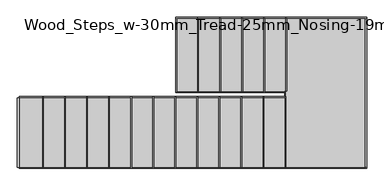
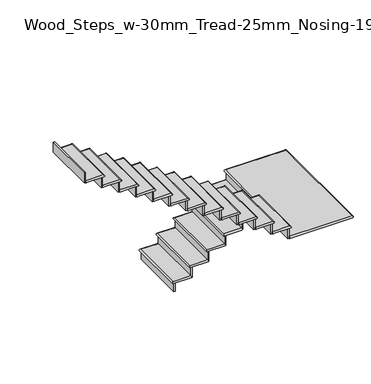
"""IFC4 building model written with IfcOpenShell, lengths in millimetres: stair flight geometry, Wood_Steps_w-30mm_Tread-25mm_Nosing-19mm_Riser."""

from ifc_helpers import new_model, si_unit, frame, origin, place, context, project, spatial, circle_curve, ellipse_curve, faceted_brep, source, transform, mapped, element, save
from ifc_brep_helpers import plane_surface, cylinder_surface, advanced_brep


def wood_steps_w_30mm_tread_25mm_nosing_19mm_riser_1d491615(model_context):
    return source(origin(), model_context, "Body", "SolidModel", [
        advanced_brep(
        [(-8665.149573, -11058.3255223, 3708.88), (-8665.149573, -11058.3255223, 3738.88), (-8665.149573, -10219.6521308, 3738.88), (-8665.149573, -10219.6521308, 3708.88), (-8400.9545789, -11058.3255223, 3738.88), (-8400.9545789, -10219.6521308, 3738.88), (-8400.9545789, -10219.6521308, 3708.88), (-8400.9545789, -11058.3255223, 3708.88)],
        [
            (0, 1, ellipse_curve(frame((-8665.149573, -11058.3255223, 3723.88), z_axis=(-0.7071067811865475, 0.7071067811865475, 0.0), x_axis=(-0.7071067811865474, -0.7071067811865476, 0.0)), 21.2132034, 15.0)),
            (1, 2),
            (2, 3, ellipse_curve(frame((-8665.149573, -10219.6521308, 3723.88), z_axis=(-0.7071067811865475, -0.7071067811865475, 0.0), x_axis=(0.7071067811865474, -0.7071067811865476, 0.0)), 21.2132034, 15.0)),
            (3, 0),
            (4, 5),
            (5, 2),
            (1, 4),
            (6, 7),
            (7, 0),
            (3, 6),
            (4, 7, circle_curve(frame((-8400.9545789, -11058.3255223, 3723.88), z_axis=(1.0, 0.0, 0.0), x_axis=(0.0, 1.0, 0.0)), 15.0)),
            (6, 5, circle_curve(frame((-8400.9545789, -10219.6521308, 3723.88), z_axis=(1.0, 0.0, 0.0), x_axis=(0.0, -1.0, 0.0)), 15.0)),
        ],
        [
            cylinder_surface(frame((-8665.149573, -11058.3255223, 3723.88), z_axis=(0.0, -1.0, 0.0), x_axis=(1.0, 0.0, 0.0)), 15.0),
            plane_surface(frame((-6495.4132565, -10219.6521308, 3738.88), z_axis=(0.0, 0.0, 1.0), x_axis=(-1.0, 0.0, 0.0))),
            plane_surface(frame((-6495.4132565, -10219.6521308, 3708.88), z_axis=(0.0, 0.0, -1.0), x_axis=(1.0, 0.0, 0.0))),
            plane_surface(frame((-8400.9545789, -11058.3255223, 3738.88), z_axis=(1.0, 0.0, 0.0), x_axis=(0.0, 0.0, -1.0))),
            cylinder_surface(frame((-8400.9545789, -11058.3255223, 3723.88), z_axis=(1.0, 0.0, 0.0), x_axis=(0.0, 1.0, 0.0)), 15.0),
            cylinder_surface(frame((-8665.149573, -10219.6521308, 3723.88), z_axis=(-1.0, 0.0, 0.0), x_axis=(0.0, -1.0, 0.0)), 15.0),
        ],
        [
            (0, [[1, 2, 3, 4]]),
            (1, [[5, 6, -2, 7]]),
            (2, [[8, 9, -4, 10]]),
            (3, [[-5, 11, -8, 12]]),
            (4, [[-11, -7, -1, -9]]),
            (5, [[-3, -6, -12, -10]]),
        ],
    ),
        faceted_brep([(-8655.149573, -11058.3255223, 3708.88), (-8655.149573, -11058.3255223, 3576.32), (-8636.149573, -11058.3255223, 3576.32), (-8636.149573, -11058.3255223, 3708.88), (-8655.149573, -10219.6521308, 3708.88), (-8636.149573, -10219.6521308, 3708.88), (-8636.149573, -10219.6521308, 3576.32), (-8655.149573, -10219.6521308, 3576.32)], [[[0, 1, 2, 3]], [[4, 5, 6, 7]], [[1, 0, 4, 7]], [[2, 1, 7, 6]], [[3, 2, 6, 5]], [[0, 3, 5, 4]]]),
        faceted_brep([(-8400.9545789, -11058.3255223, 3871.44), (-8400.9545789, -11058.3255223, 3708.88), (-8381.9545789, -11058.3255223, 3708.88), (-8381.9545789, -11058.3255223, 3871.44), (-8400.9545789, -10219.6521308, 3871.44), (-8381.9545789, -10219.6521308, 3871.44), (-8381.9545789, -10219.6521308, 3708.88), (-8400.9545789, -10219.6521308, 3708.88)], [[[0, 1, 2, 3]], [[4, 5, 6, 7]], [[1, 0, 4, 7]], [[2, 1, 7, 6]], [[3, 2, 6, 5]], [[0, 3, 5, 4]]]),
        advanced_brep(
        [(-8146.7595849, -11058.3255223, 3901.44), (-8146.7595849, -10219.6521308, 3901.44), (-8410.9545789, -10219.6521308, 3901.44), (-8410.9545789, -11058.3255223, 3901.44), (-8146.7595849, -10219.6521308, 3871.44), (-8146.7595849, -11058.3255223, 3871.44), (-8410.9545789, -11058.3255223, 3871.44), (-8410.9545789, -10219.6521308, 3871.44)],
        [
            (0, 1),
            (1, 2),
            (2, 3),
            (3, 0),
            (4, 5),
            (5, 6),
            (6, 7),
            (7, 4),
            (0, 5, circle_curve(frame((-8146.7595849, -11058.3255223, 3886.44), z_axis=(1.0, 0.0, 0.0), x_axis=(0.0, 1.0, 0.0)), 15.0)),
            (4, 1, circle_curve(frame((-8146.7595849, -10219.6521308, 3886.44), z_axis=(1.0, 0.0, 0.0), x_axis=(0.0, -1.0, 0.0)), 15.0)),
            (6, 3, ellipse_curve(frame((-8410.9545789, -11058.3255223, 3886.44), z_axis=(-0.7071067811865475, 0.7071067811865475, 0.0), x_axis=(-0.7071067811865474, -0.7071067811865476, 0.0)), 21.2132034, 15.0)),
            (2, 7, ellipse_curve(frame((-8410.9545789, -10219.6521308, 3886.44), z_axis=(-0.7071067811865475, -0.7071067811865475, 0.0), x_axis=(0.7071067811865474, -0.7071067811865476, 0.0)), 21.2132034, 15.0)),
        ],
        [
            plane_surface(frame((-6495.4132565, -10219.6521308, 3901.44), z_axis=(0.0, 0.0, 1.0), x_axis=(-1.0, 0.0, 0.0))),
            plane_surface(frame((-6495.4132565, -10219.6521308, 3871.44), z_axis=(0.0, 0.0, -1.0), x_axis=(1.0, 0.0, 0.0))),
            plane_surface(frame((-8146.7595849, -11058.3255223, 3901.44), z_axis=(1.0, 0.0, 0.0), x_axis=(0.0, 0.0, -1.0))),
            cylinder_surface(frame((-8410.9545789, -11058.3255223, 3886.44), z_axis=(0.0, -1.0, 0.0), x_axis=(1.0, 0.0, 0.0)), 15.0),
            cylinder_surface(frame((-8146.7595849, -11058.3255223, 3886.44), z_axis=(1.0, 0.0, 0.0), x_axis=(0.0, 1.0, 0.0)), 15.0),
            cylinder_surface(frame((-8410.9545789, -10219.6521308, 3886.44), z_axis=(-1.0, 0.0, 0.0), x_axis=(0.0, -1.0, 0.0)), 15.0),
        ],
        [
            (0, [[1, 2, 3, 4]]),
            (1, [[5, 6, 7, 8]]),
            (2, [[-1, 9, -5, 10]]),
            (3, [[11, -3, 12, -7]]),
            (4, [[-9, -4, -11, -6]]),
            (5, [[-12, -2, -10, -8]]),
        ],
    ),
        faceted_brep([(-8146.7595849, -11058.3255223, 4034.0), (-8146.7595849, -11058.3255223, 3871.44), (-8127.7595849, -11058.3255223, 3871.44), (-8127.7595849, -11058.3255223, 4034.0), (-8146.7595849, -10219.6521308, 4034.0), (-8127.7595849, -10219.6521308, 4034.0), (-8127.7595849, -10219.6521308, 3871.44), (-8146.7595849, -10219.6521308, 3871.44)], [[[0, 1, 2, 3]], [[4, 5, 6, 7]], [[1, 0, 4, 7]], [[2, 1, 7, 6]], [[3, 2, 6, 5]], [[0, 3, 5, 4]]]),
        advanced_brep(
        [(-7893.1206135, -11058.3255223, 4064.0), (-7893.1206135, -10219.6521308, 4064.0), (-8156.7595849, -10219.6521308, 4064.0), (-8156.7595849, -11058.3255223, 4064.0), (-7893.1206135, -10219.6521308, 4034.0), (-7893.1206135, -11058.3255223, 4034.0), (-8156.7595849, -11058.3255223, 4034.0), (-8156.7595849, -10219.6521308, 4034.0)],
        [
            (0, 1),
            (1, 2),
            (2, 3),
            (3, 0),
            (4, 5),
            (5, 6),
            (6, 7),
            (7, 4),
            (0, 5, circle_curve(frame((-7893.1206135, -11058.3255223, 4049.0), z_axis=(1.0, 0.0, 0.0), x_axis=(0.0, 1.0, 0.0)), 15.0)),
            (4, 1, circle_curve(frame((-7893.1206135, -10219.6521308, 4049.0), z_axis=(1.0, 0.0, 0.0), x_axis=(0.0, -1.0, 0.0)), 15.0)),
            (6, 3, ellipse_curve(frame((-8156.7595849, -11058.3255223, 4049.0), z_axis=(-0.7071067811865475, 0.7071067811865475, 0.0), x_axis=(-0.7071067811865474, -0.7071067811865476, 0.0)), 21.2132034, 15.0)),
            (2, 7, ellipse_curve(frame((-8156.7595849, -10219.6521308, 4049.0), z_axis=(-0.7071067811865475, -0.7071067811865475, 0.0), x_axis=(0.7071067811865474, -0.7071067811865476, 0.0)), 21.2132034, 15.0)),
        ],
        [
            plane_surface(frame((-6495.4132565, -10219.6521308, 4064.0), z_axis=(0.0, 0.0, 1.0), x_axis=(-1.0, 0.0, 0.0))),
            plane_surface(frame((-6495.4132565, -10219.6521308, 4034.0), z_axis=(0.0, 0.0, -1.0), x_axis=(1.0, 0.0, 0.0))),
            plane_surface(frame((-7893.1206135, -11058.3255223, 4064.0), z_axis=(1.0, 0.0, 0.0), x_axis=(0.0, 0.0, -1.0))),
            cylinder_surface(frame((-8156.7595849, -11058.3255223, 4049.0), z_axis=(0.0, -1.0, 0.0), x_axis=(1.0, 0.0, 0.0)), 15.0),
            cylinder_surface(frame((-7893.1206135, -11058.3255223, 4049.0), z_axis=(1.0, 0.0, 0.0), x_axis=(0.0, 1.0, 0.0)), 15.0),
            cylinder_surface(frame((-8156.7595849, -10219.6521308, 4049.0), z_axis=(-1.0, 0.0, 0.0), x_axis=(0.0, -1.0, 0.0)), 15.0),
        ],
        [
            (0, [[1, 2, 3, 4]]),
            (1, [[5, 6, 7, 8]]),
            (2, [[-1, 9, -5, 10]]),
            (3, [[11, -3, 12, -7]]),
            (4, [[-9, -4, -11, -6]]),
            (5, [[-12, -2, -10, -8]]),
        ],
    ),
        faceted_brep([(-7893.1206135, -11058.3255223, 4196.56), (-7893.1206135, -11058.3255223, 4034.0), (-7874.1206135, -11058.3255223, 4034.0), (-7874.1206135, -11058.3255223, 4196.56), (-7893.1206135, -10219.6521308, 4196.56), (-7874.1206135, -10219.6521308, 4196.56), (-7874.1206135, -10219.6521308, 4034.0), (-7893.1206135, -10219.6521308, 4034.0)], [[[0, 1, 2, 3]], [[4, 5, 6, 7]], [[1, 0, 4, 7]], [[2, 1, 7, 6]], [[3, 2, 6, 5]], [[0, 3, 5, 4]]]),
        advanced_brep(
        [(-7638.9256194, -11058.3255223, 4226.56), (-7638.9256194, -10219.6521308, 4226.56), (-7903.1206135, -10219.6521308, 4226.56), (-7903.1206135, -11058.3255223, 4226.56), (-7638.9256194, -10219.6521308, 4196.56), (-7638.9256194, -11058.3255223, 4196.56), (-7903.1206135, -11058.3255223, 4196.56), (-7903.1206135, -10219.6521308, 4196.56)],
        [
            (0, 1),
            (1, 2),
            (2, 3),
            (3, 0),
            (4, 5),
            (5, 6),
            (6, 7),
            (7, 4),
            (0, 5, circle_curve(frame((-7638.9256194, -11058.3255223, 4211.56), z_axis=(1.0, 0.0, 0.0), x_axis=(0.0, 1.0, 0.0)), 15.0)),
            (4, 1, circle_curve(frame((-7638.9256194, -10219.6521308, 4211.56), z_axis=(1.0, 0.0, 0.0), x_axis=(0.0, -1.0, 0.0)), 15.0)),
            (6, 3, ellipse_curve(frame((-7903.1206135, -11058.3255223, 4211.56), z_axis=(-0.7071067811865475, 0.7071067811865475, 0.0), x_axis=(-0.7071067811865474, -0.7071067811865476, 0.0)), 21.2132034, 15.0)),
            (2, 7, ellipse_curve(frame((-7903.1206135, -10219.6521308, 4211.56), z_axis=(-0.7071067811865475, -0.7071067811865475, 0.0), x_axis=(0.7071067811865474, -0.7071067811865476, 0.0)), 21.2132034, 15.0)),
        ],
        [
            plane_surface(frame((-6495.4132565, -10219.6521308, 4226.56), z_axis=(0.0, 0.0, 1.0), x_axis=(-1.0, 0.0, 0.0))),
            plane_surface(frame((-6495.4132565, -10219.6521308, 4196.56), z_axis=(0.0, 0.0, -1.0), x_axis=(1.0, 0.0, 0.0))),
            plane_surface(frame((-7638.9256194, -11058.3255223, 4226.56), z_axis=(1.0, 0.0, 0.0), x_axis=(0.0, 0.0, -1.0))),
            cylinder_surface(frame((-7903.1206135, -11058.3255223, 4211.56), z_axis=(0.0, -1.0, 0.0), x_axis=(1.0, 0.0, 0.0)), 15.0),
            cylinder_surface(frame((-7638.9256194, -11058.3255223, 4211.56), z_axis=(1.0, 0.0, 0.0), x_axis=(0.0, 1.0, 0.0)), 15.0),
            cylinder_surface(frame((-7903.1206135, -10219.6521308, 4211.56), z_axis=(-1.0, 0.0, 0.0), x_axis=(0.0, -1.0, 0.0)), 15.0),
        ],
        [
            (0, [[1, 2, 3, 4]]),
            (1, [[5, 6, 7, 8]]),
            (2, [[-1, 9, -5, 10]]),
            (3, [[11, -3, 12, -7]]),
            (4, [[-9, -4, -11, -6]]),
            (5, [[-12, -2, -10, -8]]),
        ],
    ),
        faceted_brep([(-7384.7306254, -11058.3255223, 4521.68), (-7384.7306254, -11058.3255223, 4359.12), (-7365.7306254, -11058.3255223, 4359.12), (-7365.7306254, -11058.3255223, 4521.68), (-7384.7306254, -10219.6521308, 4521.68), (-7365.7306254, -10219.6521308, 4521.68), (-7365.7306254, -10219.6521308, 4359.12), (-7384.7306254, -10219.6521308, 4359.12)], [[[0, 1, 2, 3]], [[4, 5, 6, 7]], [[1, 0, 4, 7]], [[2, 1, 7, 6]], [[3, 2, 6, 5]], [[0, 3, 5, 4]]]),
        faceted_brep([(-7434.7306254, -11134.5255223, 4684.24), (-7434.7306254, -11134.5255223, 4521.68), (-7453.7306254, -11134.5255223, 4521.68), (-7453.7306254, -11134.5255223, 4684.24), (-7434.7306254, -11934.0860066, 4684.24), (-7453.7306254, -11934.0860066, 4684.24), (-7453.7306254, -11934.0860066, 4521.68), (-7434.7306254, -11934.0860066, 4521.68)], [[[0, 1, 2, 3]], [[4, 5, 6, 7]], [[1, 0, 4, 7]], [[2, 1, 7, 6]], [[3, 2, 6, 5]], [[0, 3, 5, 4]]]),
        advanced_brep(
        [(-7688.9256194, -11134.5255223, 4714.24), (-7688.9256194, -11934.0860066, 4714.24), (-7424.7306254, -11934.0860066, 4714.24), (-7424.7306254, -11134.5255223, 4714.24), (-7688.9256194, -11934.0860066, 4684.24), (-7688.9256194, -11134.5255223, 4684.24), (-7424.7306254, -11134.5255223, 4684.24), (-7424.7306254, -11934.0860066, 4684.24)],
        [
            (0, 1),
            (1, 2),
            (2, 3),
            (3, 0),
            (4, 5),
            (5, 6),
            (6, 7),
            (7, 4),
            (0, 5, circle_curve(frame((-7688.9256194, -11134.5255223, 4699.24), z_axis=(-1.0, 0.0, 0.0), x_axis=(0.0, -1.0, 0.0)), 15.0)),
            (4, 1, circle_curve(frame((-7688.9256194, -11934.0860066, 4699.24), z_axis=(-1.0, 0.0, 0.0), x_axis=(0.0, 1.0, 0.0)), 15.0)),
            (6, 3, ellipse_curve(frame((-7424.7306254, -11134.5255223, 4699.24), z_axis=(0.7071067811865475, -0.7071067811865475, 0.0), x_axis=(0.7071067811865474, 0.7071067811865476, 0.0)), 21.2132034, 15.0)),
            (2, 7, ellipse_curve(frame((-7424.7306254, -11934.0860066, 4699.24), z_axis=(0.7071067811865475, 0.7071067811865475, 0.0), x_axis=(-0.7071067811865474, 0.7071067811865476, 0.0)), 21.2132034, 15.0)),
        ],
        [
            plane_surface(frame((-10457.8773536, -11934.0860066, 4714.24), z_axis=(0.0, 0.0, 1.0), x_axis=(1.0, 0.0, 0.0))),
            plane_surface(frame((-10457.8773536, -11934.0860066, 4684.24), z_axis=(0.0, 0.0, -1.0), x_axis=(-1.0, 0.0, 0.0))),
            plane_surface(frame((-7688.9256194, -11134.5255223, 4714.24), z_axis=(-1.0, 0.0, 0.0), x_axis=(0.0, 0.0, -1.0))),
            cylinder_surface(frame((-7424.7306254, -11134.5255223, 4699.24), z_axis=(0.0, 1.0, 0.0), x_axis=(-1.0, 0.0, 0.0)), 15.0),
            cylinder_surface(frame((-7688.9256194, -11134.5255223, 4699.24), z_axis=(-1.0, 0.0, 0.0), x_axis=(0.0, -1.0, 0.0)), 15.0),
            cylinder_surface(frame((-7424.7306254, -11934.0860066, 4699.24), z_axis=(1.0, 0.0, 0.0), x_axis=(0.0, 1.0, 0.0)), 15.0),
        ],
        [
            (0, [[1, 2, 3, 4]]),
            (1, [[5, 6, 7, 8]]),
            (2, [[-1, 9, -5, 10]]),
            (3, [[11, -3, 12, -7]]),
            (4, [[-9, -4, -11, -6]]),
            (5, [[-12, -2, -10, -8]]),
        ],
    ),
        faceted_brep([(-8196.7595849, -11134.5255223, 5171.92), (-8196.7595849, -11134.5255223, 5009.36), (-8215.7595849, -11134.5255223, 5009.36), (-8215.7595849, -11134.5255223, 5171.92), (-8196.7595849, -11934.0860066, 5171.92), (-8215.7595849, -11934.0860066, 5171.92), (-8215.7595849, -11934.0860066, 5009.36), (-8196.7595849, -11934.0860066, 5009.36)], [[[0, 1, 2, 3]], [[4, 5, 6, 7]], [[1, 0, 4, 7]], [[2, 1, 7, 6]], [[3, 2, 6, 5]], [[0, 3, 5, 4]]]),
        advanced_brep(
        [(-8450.9545789, -11134.5255223, 5201.92), (-8450.9545789, -11934.0860066, 5201.92), (-8186.7595849, -11934.0860066, 5201.92), (-8186.7595849, -11134.5255223, 5201.92), (-8450.9545789, -11934.0860066, 5171.92), (-8450.9545789, -11134.5255223, 5171.92), (-8186.7595849, -11134.5255223, 5171.92), (-8186.7595849, -11934.0860066, 5171.92)],
        [
            (0, 1),
            (1, 2),
            (2, 3),
            (3, 0),
            (4, 5),
            (5, 6),
            (6, 7),
            (7, 4),
            (0, 5, circle_curve(frame((-8450.9545789, -11134.5255223, 5186.92), z_axis=(-1.0, 0.0, 0.0), x_axis=(0.0, -1.0, 0.0)), 15.0)),
            (4, 1, circle_curve(frame((-8450.9545789, -11934.0860066, 5186.92), z_axis=(-1.0, 0.0, 0.0), x_axis=(0.0, 1.0, 0.0)), 15.0)),
            (6, 3, ellipse_curve(frame((-8186.7595849, -11134.5255223, 5186.92), z_axis=(0.7071067811865475, -0.7071067811865475, 0.0), x_axis=(0.7071067811865474, 0.7071067811865476, 0.0)), 21.2132034, 15.0)),
            (2, 7, ellipse_curve(frame((-8186.7595849, -11934.0860066, 5186.92), z_axis=(0.7071067811865475, 0.7071067811865475, 0.0), x_axis=(-0.7071067811865474, 0.7071067811865476, 0.0)), 21.2132034, 15.0)),
        ],
        [
            plane_surface(frame((-10457.8773536, -11934.0860066, 5201.92), z_axis=(0.0, 0.0, 1.0), x_axis=(1.0, 0.0, 0.0))),
            plane_surface(frame((-10457.8773536, -11934.0860066, 5171.92), z_axis=(0.0, 0.0, -1.0), x_axis=(-1.0, 0.0, 0.0))),
            plane_surface(frame((-8450.9545789, -11134.5255223, 5201.92), z_axis=(-1.0, 0.0, 0.0), x_axis=(0.0, 0.0, -1.0))),
            cylinder_surface(frame((-8186.7595849, -11134.5255223, 5186.92), z_axis=(0.0, 1.0, 0.0), x_axis=(-1.0, 0.0, 0.0)), 15.0),
            cylinder_surface(frame((-8450.9545789, -11134.5255223, 5186.92), z_axis=(-1.0, 0.0, 0.0), x_axis=(0.0, -1.0, 0.0)), 15.0),
            cylinder_surface(frame((-8186.7595849, -11934.0860066, 5186.92), z_axis=(1.0, 0.0, 0.0), x_axis=(0.0, 1.0, 0.0)), 15.0),
        ],
        [
            (0, [[1, 2, 3, 4]]),
            (1, [[5, 6, 7, 8]]),
            (2, [[-1, 9, -5, 10]]),
            (3, [[11, -3, 12, -7]]),
            (4, [[-9, -4, -11, -6]]),
            (5, [[-12, -2, -10, -8]]),
        ],
    ),
        faceted_brep([(-8958.7885444, -11134.5255223, 5659.6), (-8958.7885444, -11134.5255223, 5497.04), (-8977.7885444, -11134.5255223, 5497.04), (-8977.7885444, -11134.5255223, 5659.6), (-8958.7885444, -11934.0860066, 5659.6), (-8977.7885444, -11934.0860066, 5659.6), (-8977.7885444, -11934.0860066, 5497.04), (-8958.7885444, -11934.0860066, 5497.04)], [[[0, 1, 2, 3]], [[4, 5, 6, 7]], [[1, 0, 4, 7]], [[2, 1, 7, 6]], [[3, 2, 6, 5]], [[0, 3, 5, 4]]]),
        advanced_brep(
        [(-9212.9835384, -11134.5255223, 5689.6), (-9212.9835384, -11934.0860066, 5689.6), (-8948.7885444, -11934.0860066, 5689.6), (-8948.7885444, -11134.5255223, 5689.6), (-9212.9835384, -11934.0860066, 5659.6), (-9212.9835384, -11134.5255223, 5659.6), (-8948.7885444, -11134.5255223, 5659.6), (-8948.7885444, -11934.0860066, 5659.6)],
        [
            (0, 1),
            (1, 2),
            (2, 3),
            (3, 0),
            (4, 5),
            (5, 6),
            (6, 7),
            (7, 4),
            (0, 5, circle_curve(frame((-9212.9835384, -11134.5255223, 5674.6), z_axis=(-1.0, 0.0, 0.0), x_axis=(0.0, -1.0, 0.0)), 15.0)),
            (4, 1, circle_curve(frame((-9212.9835384, -11934.0860066, 5674.6), z_axis=(-1.0, 0.0, 0.0), x_axis=(0.0, 1.0, 0.0)), 15.0)),
            (6, 3, ellipse_curve(frame((-8948.7885444, -11134.5255223, 5674.6), z_axis=(0.7071067811865475, -0.7071067811865475, 0.0), x_axis=(0.7071067811865474, 0.7071067811865476, 0.0)), 21.2132034, 15.0)),
            (2, 7, ellipse_curve(frame((-8948.7885444, -11934.0860066, 5674.6), z_axis=(0.7071067811865475, 0.7071067811865475, 0.0), x_axis=(-0.7071067811865474, 0.7071067811865476, 0.0)), 21.2132034, 15.0)),
        ],
        [
            plane_surface(frame((-10457.8773536, -11934.0860066, 5689.6), z_axis=(0.0, 0.0, 1.0), x_axis=(1.0, 0.0, 0.0))),
            plane_surface(frame((-10457.8773536, -11934.0860066, 5659.6), z_axis=(0.0, 0.0, -1.0), x_axis=(-1.0, 0.0, 0.0))),
            plane_surface(frame((-9212.9835384, -11134.5255223, 5689.6), z_axis=(-1.0, 0.0, 0.0), x_axis=(0.0, 0.0, -1.0))),
            cylinder_surface(frame((-8948.7885444, -11134.5255223, 5674.6), z_axis=(0.0, 1.0, 0.0), x_axis=(-1.0, 0.0, 0.0)), 15.0),
            cylinder_surface(frame((-9212.9835384, -11134.5255223, 5674.6), z_axis=(-1.0, 0.0, 0.0), x_axis=(0.0, -1.0, 0.0)), 15.0),
            cylinder_surface(frame((-8948.7885444, -11934.0860066, 5674.6), z_axis=(1.0, 0.0, 0.0), x_axis=(0.0, 1.0, 0.0)), 15.0),
        ],
        [
            (0, [[1, 2, 3, 4]]),
            (1, [[5, 6, 7, 8]]),
            (2, [[-1, 9, -5, 10]]),
            (3, [[11, -3, 12, -7]]),
            (4, [[-9, -4, -11, -6]]),
            (5, [[-12, -2, -10, -8]]),
        ],
    ),
        faceted_brep([(-9212.9835384, -11134.5255223, 5822.16), (-9212.9835384, -11134.5255223, 5659.6), (-9231.9835384, -11134.5255223, 5659.6), (-9231.9835384, -11134.5255223, 5822.16), (-9212.9835384, -11934.0860066, 5822.16), (-9231.9835384, -11934.0860066, 5822.16), (-9231.9835384, -11934.0860066, 5659.6), (-9212.9835384, -11934.0860066, 5659.6)], [[[0, 1, 2, 3]], [[4, 5, 6, 7]], [[1, 0, 4, 7]], [[2, 1, 7, 6]], [[3, 2, 6, 5]], [[0, 3, 5, 4]]]),
        advanced_brep(
        [(-9466.6534, -11134.5255223, 5852.16), (-9466.6534, -11934.0860066, 5852.16), (-9202.9835384, -11934.0860066, 5852.16), (-9202.9835384, -11134.5255223, 5852.16), (-9466.6534, -11934.0860066, 5822.16), (-9466.6534, -11134.5255223, 5822.16), (-9202.9835384, -11134.5255223, 5822.16), (-9202.9835384, -11934.0860066, 5822.16)],
        [
            (0, 1),
            (1, 2),
            (2, 3),
            (3, 0),
            (4, 5),
            (5, 6),
            (6, 7),
            (7, 4),
            (0, 5, circle_curve(frame((-9466.6534, -11134.5255223, 5837.16), z_axis=(-1.0, 0.0, 0.0), x_axis=(0.0, -1.0, 0.0)), 15.0)),
            (4, 1, circle_curve(frame((-9466.6534, -11934.0860066, 5837.16), z_axis=(-1.0, 0.0, 0.0), x_axis=(0.0, 1.0, 0.0)), 15.0)),
            (6, 3, ellipse_curve(frame((-9202.9835384, -11134.5255223, 5837.16), z_axis=(0.7071067811865475, -0.7071067811865475, 0.0), x_axis=(0.7071067811865474, 0.7071067811865476, 0.0)), 21.2132034, 15.0)),
            (2, 7, ellipse_curve(frame((-9202.9835384, -11934.0860066, 5837.16), z_axis=(0.7071067811865475, 0.7071067811865475, 0.0), x_axis=(-0.7071067811865474, 0.7071067811865476, 0.0)), 21.2132034, 15.0)),
        ],
        [
            plane_surface(frame((-10457.8773536, -11934.0860066, 5852.16), z_axis=(0.0, 0.0, 1.0), x_axis=(1.0, 0.0, 0.0))),
            plane_surface(frame((-10457.8773536, -11934.0860066, 5822.16), z_axis=(0.0, 0.0, -1.0), x_axis=(-1.0, 0.0, 0.0))),
            plane_surface(frame((-9466.6534, -11134.5255223, 5852.16), z_axis=(-1.0, 0.0, 0.0), x_axis=(0.0, 0.0, -1.0))),
            cylinder_surface(frame((-9202.9835384, -11134.5255223, 5837.16), z_axis=(0.0, 1.0, 0.0), x_axis=(-1.0, 0.0, 0.0)), 15.0),
            cylinder_surface(frame((-9466.6534, -11134.5255223, 5837.16), z_axis=(-1.0, 0.0, 0.0), x_axis=(0.0, -1.0, 0.0)), 15.0),
            cylinder_surface(frame((-9202.9835384, -11934.0860066, 5837.16), z_axis=(1.0, 0.0, 0.0), x_axis=(0.0, 1.0, 0.0)), 15.0),
        ],
        [
            (0, [[1, 2, 3, 4]]),
            (1, [[5, 6, 7, 8]]),
            (2, [[-1, 9, -5, 10]]),
            (3, [[11, -3, 12, -7]]),
            (4, [[-9, -4, -11, -6]]),
            (5, [[-12, -2, -10, -8]]),
        ],
    ),
        faceted_brep([(-9720.8175039, -11134.5255223, 6147.28), (-9720.8175039, -11134.5255223, 5984.72), (-9739.8175039, -11134.5255223, 5984.72), (-9739.8175039, -11134.5255223, 6147.28), (-9720.8175039, -11934.0860066, 6147.28), (-9739.8175039, -11934.0860066, 6147.28), (-9739.8175039, -11934.0860066, 5984.72), (-9720.8175039, -11934.0860066, 5984.72)], [[[0, 1, 2, 3]], [[4, 5, 6, 7]], [[1, 0, 4, 7]], [[2, 1, 7, 6]], [[3, 2, 6, 5]], [[0, 3, 5, 4]]]),
        advanced_brep(
        [(-9975.012498, -11134.5255223, 6177.28), (-9975.012498, -11934.0860066, 6177.28), (-9710.8175039, -11934.0860066, 6177.28), (-9710.8175039, -11134.5255223, 6177.28), (-9975.012498, -11934.0860066, 6147.28), (-9975.012498, -11134.5255223, 6147.28), (-9710.8175039, -11134.5255223, 6147.28), (-9710.8175039, -11934.0860066, 6147.28)],
        [
            (0, 1),
            (1, 2),
            (2, 3),
            (3, 0),
            (4, 5),
            (5, 6),
            (6, 7),
            (7, 4),
            (0, 5, circle_curve(frame((-9975.012498, -11134.5255223, 6162.28), z_axis=(-1.0, 0.0, 0.0), x_axis=(0.0, -1.0, 0.0)), 15.0)),
            (4, 1, circle_curve(frame((-9975.012498, -11934.0860066, 6162.28), z_axis=(-1.0, 0.0, 0.0), x_axis=(0.0, 1.0, 0.0)), 15.0)),
            (6, 3, ellipse_curve(frame((-9710.8175039, -11134.5255223, 6162.28), z_axis=(0.7071067811865475, -0.7071067811865475, 0.0), x_axis=(0.7071067811865474, 0.7071067811865476, 0.0)), 21.2132034, 15.0)),
            (2, 7, ellipse_curve(frame((-9710.8175039, -11934.0860066, 6162.28), z_axis=(0.7071067811865475, 0.7071067811865475, 0.0), x_axis=(-0.7071067811865474, 0.7071067811865476, 0.0)), 21.2132034, 15.0)),
        ],
        [
            plane_surface(frame((-10457.8773536, -11934.0860066, 6177.28), z_axis=(0.0, 0.0, 1.0), x_axis=(1.0, 0.0, 0.0))),
            plane_surface(frame((-10457.8773536, -11934.0860066, 6147.28), z_axis=(0.0, 0.0, -1.0), x_axis=(-1.0, 0.0, 0.0))),
            plane_surface(frame((-9975.012498, -11134.5255223, 6177.28), z_axis=(-1.0, 0.0, 0.0), x_axis=(0.0, 0.0, -1.0))),
            cylinder_surface(frame((-9710.8175039, -11134.5255223, 6162.28), z_axis=(0.0, 1.0, 0.0), x_axis=(-1.0, 0.0, 0.0)), 15.0),
            cylinder_surface(frame((-9975.012498, -11134.5255223, 6162.28), z_axis=(-1.0, 0.0, 0.0), x_axis=(0.0, -1.0, 0.0)), 15.0),
            cylinder_surface(frame((-9710.8175039, -11934.0860066, 6162.28), z_axis=(1.0, 0.0, 0.0), x_axis=(0.0, 1.0, 0.0)), 15.0),
        ],
        [
            (0, [[1, 2, 3, 4]]),
            (1, [[5, 6, 7, 8]]),
            (2, [[-1, 9, -5, 10]]),
            (3, [[11, -3, 12, -7]]),
            (4, [[-9, -4, -11, -6]]),
            (5, [[-12, -2, -10, -8]]),
        ],
    ),
        faceted_brep([(-9975.012498, -11134.5255223, 6309.84), (-9975.012498, -11134.5255223, 6147.28), (-9994.012498, -11134.5255223, 6147.28), (-9994.012498, -11134.5255223, 6309.84), (-9975.012498, -11934.0860066, 6309.84), (-9994.012498, -11934.0860066, 6309.84), (-9994.012498, -11934.0860066, 6147.28), (-9975.012498, -11934.0860066, 6147.28)], [[[0, 1, 2, 3]], [[4, 5, 6, 7]], [[1, 0, 4, 7]], [[2, 1, 7, 6]], [[3, 2, 6, 5]], [[0, 3, 5, 4]]]),
        advanced_brep(
        [(-10228.6823595, -11134.5255223, 6339.84), (-10228.6823595, -11934.0860066, 6339.84), (-9965.012498, -11934.0860066, 6339.84), (-9965.012498, -11134.5255223, 6339.84), (-10228.6823595, -11934.0860066, 6309.84), (-10228.6823595, -11134.5255223, 6309.84), (-9965.012498, -11134.5255223, 6309.84), (-9965.012498, -11934.0860066, 6309.84)],
        [
            (0, 1),
            (1, 2),
            (2, 3),
            (3, 0),
            (4, 5),
            (5, 6),
            (6, 7),
            (7, 4),
            (0, 5, circle_curve(frame((-10228.6823595, -11134.5255223, 6324.84), z_axis=(-1.0, 0.0, 0.0), x_axis=(0.0, -1.0, 0.0)), 15.0)),
            (4, 1, circle_curve(frame((-10228.6823595, -11934.0860066, 6324.84), z_axis=(-1.0, 0.0, 0.0), x_axis=(0.0, 1.0, 0.0)), 15.0)),
            (6, 3, ellipse_curve(frame((-9965.012498, -11134.5255223, 6324.84), z_axis=(0.7071067811865475, -0.7071067811865475, 0.0), x_axis=(0.7071067811865474, 0.7071067811865476, 0.0)), 21.2132034, 15.0)),
            (2, 7, ellipse_curve(frame((-9965.012498, -11934.0860066, 6324.84), z_axis=(0.7071067811865475, 0.7071067811865475, 0.0), x_axis=(-0.7071067811865474, 0.7071067811865476, 0.0)), 21.2132034, 15.0)),
        ],
        [
            plane_surface(frame((-10457.8773536, -11934.0860066, 6339.84), z_axis=(0.0, 0.0, 1.0), x_axis=(1.0, 0.0, 0.0))),
            plane_surface(frame((-10457.8773536, -11934.0860066, 6309.84), z_axis=(0.0, 0.0, -1.0), x_axis=(-1.0, 0.0, 0.0))),
            plane_surface(frame((-10228.6823595, -11134.5255223, 6339.84), z_axis=(-1.0, 0.0, 0.0), x_axis=(0.0, 0.0, -1.0))),
            cylinder_surface(frame((-9965.012498, -11134.5255223, 6324.84), z_axis=(0.0, 1.0, 0.0), x_axis=(-1.0, 0.0, 0.0)), 15.0),
            cylinder_surface(frame((-10228.6823595, -11134.5255223, 6324.84), z_axis=(-1.0, 0.0, 0.0), x_axis=(0.0, -1.0, 0.0)), 15.0),
            cylinder_surface(frame((-9965.012498, -11934.0860066, 6324.84), z_axis=(1.0, 0.0, 0.0), x_axis=(0.0, 1.0, 0.0)), 15.0),
        ],
        [
            (0, [[1, 2, 3, 4]]),
            (1, [[5, 6, 7, 8]]),
            (2, [[-1, 9, -5, 10]]),
            (3, [[11, -3, 12, -7]]),
            (4, [[-9, -4, -11, -6]]),
            (5, [[-12, -2, -10, -8]]),
        ],
    ),
        faceted_brep([(-10482.8773536, -11134.5255223, 6634.96), (-10482.8773536, -11134.5255223, 6472.4), (-10501.8773536, -11134.5255223, 6472.4), (-10501.8773536, -11134.5255223, 6634.96), (-10482.8773536, -11934.0860066, 6634.96), (-10501.8773536, -11934.0860066, 6634.96), (-10501.8773536, -11934.0860066, 6472.4), (-10482.8773536, -11934.0860066, 6472.4)], [[[0, 1, 2, 3]], [[4, 5, 6, 7]], [[1, 0, 4, 7]], [[2, 1, 7, 6]], [[3, 2, 6, 5]], [[0, 3, 5, 4]]]),
        faceted_brep([(-7638.9256194, -11058.3255223, 4359.12), (-7638.9256194, -11058.3255223, 4196.56), (-7619.9256194, -11058.3255223, 4196.56), (-7619.9256194, -11058.3255223, 4359.12), (-7638.9256194, -10219.6521308, 4359.12), (-7619.9256194, -10219.6521308, 4359.12), (-7619.9256194, -10219.6521308, 4196.56), (-7638.9256194, -10219.6521308, 4196.56)], [[[0, 1, 2, 3]], [[4, 5, 6, 7]], [[1, 0, 4, 7]], [[2, 1, 7, 6]], [[3, 2, 6, 5]], [[0, 3, 5, 4]]]),
        advanced_brep(
        [(-7384.7306254, -11058.3255223, 4389.12), (-7384.7306254, -10219.6521308, 4389.12), (-7648.9256194, -10219.6521308, 4389.12), (-7648.9256194, -11058.3255223, 4389.12), (-7384.7306254, -10219.6521308, 4359.12), (-7384.7306254, -11058.3255223, 4359.12), (-7648.9256194, -11058.3255223, 4359.12), (-7648.9256194, -10219.6521308, 4359.12)],
        [
            (0, 1),
            (1, 2),
            (2, 3),
            (3, 0),
            (4, 5),
            (5, 6),
            (6, 7),
            (7, 4),
            (0, 5, circle_curve(frame((-7384.7306254, -11058.3255223, 4374.12), z_axis=(1.0, 0.0, 0.0), x_axis=(0.0, 1.0, 0.0)), 15.0)),
            (4, 1, circle_curve(frame((-7384.7306254, -10219.6521308, 4374.12), z_axis=(1.0, 0.0, 0.0), x_axis=(0.0, -1.0, 0.0)), 15.0)),
            (6, 3, ellipse_curve(frame((-7648.9256194, -11058.3255223, 4374.12), z_axis=(-0.7071067811865475, 0.7071067811865475, 0.0), x_axis=(-0.7071067811865474, -0.7071067811865476, 0.0)), 21.2132034, 15.0)),
            (2, 7, ellipse_curve(frame((-7648.9256194, -10219.6521308, 4374.12), z_axis=(-0.7071067811865475, -0.7071067811865475, 0.0), x_axis=(0.7071067811865474, -0.7071067811865476, 0.0)), 21.2132034, 15.0)),
        ],
        [
            plane_surface(frame((-6241.2182625, -10219.6521308, 4389.12), z_axis=(0.0, 0.0, 1.0), x_axis=(-1.0, 0.0, 0.0))),
            plane_surface(frame((-6241.2182625, -10219.6521308, 4359.12), z_axis=(0.0, 0.0, -1.0), x_axis=(1.0, 0.0, 0.0))),
            plane_surface(frame((-7384.7306254, -11058.3255223, 4389.12), z_axis=(1.0, 0.0, 0.0), x_axis=(0.0, 0.0, -1.0))),
            cylinder_surface(frame((-7648.9256194, -11058.3255223, 4374.12), z_axis=(0.0, -1.0, 0.0), x_axis=(1.0, 0.0, 0.0)), 15.0),
            cylinder_surface(frame((-7384.7306254, -11058.3255223, 4374.12), z_axis=(1.0, 0.0, 0.0), x_axis=(0.0, 1.0, 0.0)), 15.0),
            cylinder_surface(frame((-7648.9256194, -10219.6521308, 4374.12), z_axis=(-1.0, 0.0, 0.0), x_axis=(0.0, -1.0, 0.0)), 15.0),
        ],
        [
            (0, [[1, 2, 3, 4]]),
            (1, [[5, 6, 7, 8]]),
            (2, [[-1, 9, -5, 10]]),
            (3, [[11, -3, 12, -7]]),
            (4, [[-9, -4, -11, -6]]),
            (5, [[-12, -2, -10, -8]]),
        ],
    ),
        faceted_brep([(-7688.9256194, -11134.5255223, 4846.8), (-7688.9256194, -11134.5255223, 4684.24), (-7707.9256194, -11134.5255223, 4684.24), (-7707.9256194, -11134.5255223, 4846.8), (-7688.9256194, -11934.0860066, 4846.8), (-7707.9256194, -11934.0860066, 4846.8), (-7707.9256194, -11934.0860066, 4684.24), (-7688.9256194, -11934.0860066, 4684.24)], [[[0, 1, 2, 3]], [[4, 5, 6, 7]], [[1, 0, 4, 7]], [[2, 1, 7, 6]], [[3, 2, 6, 5]], [[0, 3, 5, 4]]]),
        advanced_brep(
        [(-7943.1206135, -11134.5255223, 4876.8), (-7943.1206135, -11934.0860066, 4876.8), (-7678.9256194, -11934.0860066, 4876.8), (-7678.9256194, -11134.5255223, 4876.8), (-7943.1206135, -11934.0860066, 4846.8), (-7943.1206135, -11134.5255223, 4846.8), (-7678.9256194, -11134.5255223, 4846.8), (-7678.9256194, -11934.0860066, 4846.8)],
        [
            (0, 1),
            (1, 2),
            (2, 3),
            (3, 0),
            (4, 5),
            (5, 6),
            (6, 7),
            (7, 4),
            (0, 5, circle_curve(frame((-7943.1206135, -11134.5255223, 4861.8), z_axis=(-1.0, 0.0, 0.0), x_axis=(0.0, -1.0, 0.0)), 15.0)),
            (4, 1, circle_curve(frame((-7943.1206135, -11934.0860066, 4861.8), z_axis=(-1.0, 0.0, 0.0), x_axis=(0.0, 1.0, 0.0)), 15.0)),
            (6, 3, ellipse_curve(frame((-7678.9256194, -11134.5255223, 4861.8), z_axis=(0.7071067811865475, -0.7071067811865475, 0.0), x_axis=(0.7071067811865474, 0.7071067811865476, 0.0)), 21.2132034, 15.0)),
            (2, 7, ellipse_curve(frame((-7678.9256194, -11934.0860066, 4861.8), z_axis=(0.7071067811865475, 0.7071067811865475, 0.0), x_axis=(-0.7071067811865474, 0.7071067811865476, 0.0)), 21.2132034, 15.0)),
        ],
        [
            plane_surface(frame((-10712.0723476, -11934.0860066, 4876.8), z_axis=(0.0, 0.0, 1.0), x_axis=(1.0, 0.0, 0.0))),
            plane_surface(frame((-10712.0723476, -11934.0860066, 4846.8), z_axis=(0.0, 0.0, -1.0), x_axis=(-1.0, 0.0, 0.0))),
            plane_surface(frame((-7943.1206135, -11134.5255223, 4876.8), z_axis=(-1.0, 0.0, 0.0), x_axis=(0.0, 0.0, -1.0))),
            cylinder_surface(frame((-7678.9256194, -11134.5255223, 4861.8), z_axis=(0.0, 1.0, 0.0), x_axis=(-1.0, 0.0, 0.0)), 15.0),
            cylinder_surface(frame((-7943.1206135, -11134.5255223, 4861.8), z_axis=(-1.0, 0.0, 0.0), x_axis=(0.0, -1.0, 0.0)), 15.0),
            cylinder_surface(frame((-7678.9256194, -11934.0860066, 4861.8), z_axis=(1.0, 0.0, 0.0), x_axis=(0.0, 1.0, 0.0)), 15.0),
        ],
        [
            (0, [[1, 2, 3, 4]]),
            (1, [[5, 6, 7, 8]]),
            (2, [[-1, 9, -5, 10]]),
            (3, [[11, -3, 12, -7]]),
            (4, [[-9, -4, -11, -6]]),
            (5, [[-12, -2, -10, -8]]),
        ],
    ),
        faceted_brep([(-7943.1206135, -11134.5255223, 5009.36), (-7943.1206135, -11134.5255223, 4846.8), (-7962.1206135, -11134.5255223, 4846.8), (-7962.1206135, -11134.5255223, 5009.36), (-7943.1206135, -11934.0860066, 5009.36), (-7962.1206135, -11934.0860066, 5009.36), (-7962.1206135, -11934.0860066, 4846.8), (-7943.1206135, -11934.0860066, 4846.8)], [[[0, 1, 2, 3]], [[4, 5, 6, 7]], [[1, 0, 4, 7]], [[2, 1, 7, 6]], [[3, 2, 6, 5]], [[0, 3, 5, 4]]]),
        advanced_brep(
        [(-8196.7595849, -11134.5255223, 5039.36), (-8196.7595849, -11934.0860066, 5039.36), (-7933.1206135, -11934.0860066, 5039.36), (-7933.1206135, -11134.5255223, 5039.36), (-8196.7595849, -11934.0860066, 5009.36), (-8196.7595849, -11134.5255223, 5009.36), (-7933.1206135, -11134.5255223, 5009.36), (-7933.1206135, -11934.0860066, 5009.36)],
        [
            (0, 1),
            (1, 2),
            (2, 3),
            (3, 0),
            (4, 5),
            (5, 6),
            (6, 7),
            (7, 4),
            (0, 5, circle_curve(frame((-8196.7595849, -11134.5255223, 5024.36), z_axis=(-1.0, 0.0, 0.0), x_axis=(0.0, -1.0, 0.0)), 15.0)),
            (4, 1, circle_curve(frame((-8196.7595849, -11934.0860066, 5024.36), z_axis=(-1.0, 0.0, 0.0), x_axis=(0.0, 1.0, 0.0)), 15.0)),
            (6, 3, ellipse_curve(frame((-7933.1206135, -11134.5255223, 5024.36), z_axis=(0.7071067811865475, -0.7071067811865475, 0.0), x_axis=(0.7071067811865474, 0.7071067811865476, 0.0)), 21.2132034, 15.0)),
            (2, 7, ellipse_curve(frame((-7933.1206135, -11934.0860066, 5024.36), z_axis=(0.7071067811865475, 0.7071067811865475, 0.0), x_axis=(-0.7071067811865474, 0.7071067811865476, 0.0)), 21.2132034, 15.0)),
        ],
        [
            plane_surface(frame((-10457.8773536, -11934.0860066, 5039.36), z_axis=(0.0, 0.0, 1.0), x_axis=(1.0, 0.0, 0.0))),
            plane_surface(frame((-10457.8773536, -11934.0860066, 5009.36), z_axis=(0.0, 0.0, -1.0), x_axis=(-1.0, 0.0, 0.0))),
            plane_surface(frame((-8196.7595849, -11134.5255223, 5039.36), z_axis=(-1.0, 0.0, 0.0), x_axis=(0.0, 0.0, -1.0))),
            cylinder_surface(frame((-7933.1206135, -11134.5255223, 5024.36), z_axis=(0.0, 1.0, 0.0), x_axis=(-1.0, 0.0, 0.0)), 15.0),
            cylinder_surface(frame((-8196.7595849, -11134.5255223, 5024.36), z_axis=(-1.0, 0.0, 0.0), x_axis=(0.0, -1.0, 0.0)), 15.0),
            cylinder_surface(frame((-7933.1206135, -11934.0860066, 5024.36), z_axis=(1.0, 0.0, 0.0), x_axis=(0.0, 1.0, 0.0)), 15.0),
        ],
        [
            (0, [[1, 2, 3, 4]]),
            (1, [[5, 6, 7, 8]]),
            (2, [[-1, 9, -5, 10]]),
            (3, [[11, -3, 12, -7]]),
            (4, [[-9, -4, -11, -6]]),
            (5, [[-12, -2, -10, -8]]),
        ],
    ),
        faceted_brep([(-8450.9545789, -11134.5255223, 5334.48), (-8450.9545789, -11134.5255223, 5171.92), (-8469.9545789, -11134.5255223, 5171.92), (-8469.9545789, -11134.5255223, 5334.48), (-8450.9545789, -11934.0860066, 5334.48), (-8469.9545789, -11934.0860066, 5334.48), (-8469.9545789, -11934.0860066, 5171.92), (-8450.9545789, -11934.0860066, 5171.92)], [[[0, 1, 2, 3]], [[4, 5, 6, 7]], [[1, 0, 4, 7]], [[2, 1, 7, 6]], [[3, 2, 6, 5]], [[0, 3, 5, 4]]]),
        advanced_brep(
        [(-8705.149573, -11134.5255223, 5364.48), (-8705.149573, -11934.0860066, 5364.48), (-8440.9545789, -11934.0860066, 5364.48), (-8440.9545789, -11134.5255223, 5364.48), (-8705.149573, -11934.0860066, 5334.48), (-8705.149573, -11134.5255223, 5334.48), (-8440.9545789, -11134.5255223, 5334.48), (-8440.9545789, -11934.0860066, 5334.48)],
        [
            (0, 1),
            (1, 2),
            (2, 3),
            (3, 0),
            (4, 5),
            (5, 6),
            (6, 7),
            (7, 4),
            (0, 5, circle_curve(frame((-8705.149573, -11134.5255223, 5349.48), z_axis=(-1.0, 0.0, 0.0), x_axis=(0.0, -1.0, 0.0)), 15.0)),
            (4, 1, circle_curve(frame((-8705.149573, -11934.0860066, 5349.48), z_axis=(-1.0, 0.0, 0.0), x_axis=(0.0, 1.0, 0.0)), 15.0)),
            (6, 3, ellipse_curve(frame((-8440.9545789, -11134.5255223, 5349.48), z_axis=(0.7071067811865475, -0.7071067811865475, 0.0), x_axis=(0.7071067811865474, 0.7071067811865476, 0.0)), 21.2132034, 15.0)),
            (2, 7, ellipse_curve(frame((-8440.9545789, -11934.0860066, 5349.48), z_axis=(0.7071067811865475, 0.7071067811865475, 0.0), x_axis=(-0.7071067811865474, 0.7071067811865476, 0.0)), 21.2132034, 15.0)),
        ],
        [
            plane_surface(frame((-10712.0723476, -11934.0860066, 5364.48), z_axis=(0.0, 0.0, 1.0), x_axis=(1.0, 0.0, 0.0))),
            plane_surface(frame((-10712.0723476, -11934.0860066, 5334.48), z_axis=(0.0, 0.0, -1.0), x_axis=(-1.0, 0.0, 0.0))),
            plane_surface(frame((-8705.149573, -11134.5255223, 5364.48), z_axis=(-1.0, 0.0, 0.0), x_axis=(0.0, 0.0, -1.0))),
            cylinder_surface(frame((-8440.9545789, -11134.5255223, 5349.48), z_axis=(0.0, 1.0, 0.0), x_axis=(-1.0, 0.0, 0.0)), 15.0),
            cylinder_surface(frame((-8705.149573, -11134.5255223, 5349.48), z_axis=(-1.0, 0.0, 0.0), x_axis=(0.0, -1.0, 0.0)), 15.0),
            cylinder_surface(frame((-8440.9545789, -11934.0860066, 5349.48), z_axis=(1.0, 0.0, 0.0), x_axis=(0.0, 1.0, 0.0)), 15.0),
        ],
        [
            (0, [[1, 2, 3, 4]]),
            (1, [[5, 6, 7, 8]]),
            (2, [[-1, 9, -5, 10]]),
            (3, [[11, -3, 12, -7]]),
            (4, [[-9, -4, -11, -6]]),
            (5, [[-12, -2, -10, -8]]),
        ],
    ),
        faceted_brep([(-8705.149573, -11134.5255223, 5497.04), (-8705.149573, -11134.5255223, 5334.48), (-8724.149573, -11134.5255223, 5334.48), (-8724.149573, -11134.5255223, 5497.04), (-8705.149573, -11934.0860066, 5497.04), (-8724.149573, -11934.0860066, 5497.04), (-8724.149573, -11934.0860066, 5334.48), (-8705.149573, -11934.0860066, 5334.48)], [[[0, 1, 2, 3]], [[4, 5, 6, 7]], [[1, 0, 4, 7]], [[2, 1, 7, 6]], [[3, 2, 6, 5]], [[0, 3, 5, 4]]]),
        advanced_brep(
        [(-8958.7885444, -11134.5255223, 5527.04), (-8958.7885444, -11934.0860066, 5527.04), (-8695.149573, -11934.0860066, 5527.04), (-8695.149573, -11134.5255223, 5527.04), (-8958.7885444, -11934.0860066, 5497.04), (-8958.7885444, -11134.5255223, 5497.04), (-8695.149573, -11134.5255223, 5497.04), (-8695.149573, -11934.0860066, 5497.04)],
        [
            (0, 1),
            (1, 2),
            (2, 3),
            (3, 0),
            (4, 5),
            (5, 6),
            (6, 7),
            (7, 4),
            (0, 5, circle_curve(frame((-8958.7885444, -11134.5255223, 5512.04), z_axis=(-1.0, 0.0, 0.0), x_axis=(0.0, -1.0, 0.0)), 15.0)),
            (4, 1, circle_curve(frame((-8958.7885444, -11934.0860066, 5512.04), z_axis=(-1.0, 0.0, 0.0), x_axis=(0.0, 1.0, 0.0)), 15.0)),
            (6, 3, ellipse_curve(frame((-8695.149573, -11134.5255223, 5512.04), z_axis=(0.7071067811865475, -0.7071067811865475, 0.0), x_axis=(0.7071067811865474, 0.7071067811865476, 0.0)), 21.2132034, 15.0)),
            (2, 7, ellipse_curve(frame((-8695.149573, -11934.0860066, 5512.04), z_axis=(0.7071067811865475, 0.7071067811865475, 0.0), x_axis=(-0.7071067811865474, 0.7071067811865476, 0.0)), 21.2132034, 15.0)),
        ],
        [
            plane_surface(frame((-10457.8773536, -11934.0860066, 5527.04), z_axis=(0.0, 0.0, 1.0), x_axis=(1.0, 0.0, 0.0))),
            plane_surface(frame((-10457.8773536, -11934.0860066, 5497.04), z_axis=(0.0, 0.0, -1.0), x_axis=(-1.0, 0.0, 0.0))),
            plane_surface(frame((-8958.7885444, -11134.5255223, 5527.04), z_axis=(-1.0, 0.0, 0.0), x_axis=(0.0, 0.0, -1.0))),
            cylinder_surface(frame((-8695.149573, -11134.5255223, 5512.04), z_axis=(0.0, 1.0, 0.0), x_axis=(-1.0, 0.0, 0.0)), 15.0),
            cylinder_surface(frame((-8958.7885444, -11134.5255223, 5512.04), z_axis=(-1.0, 0.0, 0.0), x_axis=(0.0, -1.0, 0.0)), 15.0),
            cylinder_surface(frame((-8695.149573, -11934.0860066, 5512.04), z_axis=(1.0, 0.0, 0.0), x_axis=(0.0, 1.0, 0.0)), 15.0),
        ],
        [
            (0, [[1, 2, 3, 4]]),
            (1, [[5, 6, 7, 8]]),
            (2, [[-1, 9, -5, 10]]),
            (3, [[11, -3, 12, -7]]),
            (4, [[-9, -4, -11, -6]]),
            (5, [[-12, -2, -10, -8]]),
        ],
    ),
        faceted_brep([(-9466.6534, -11134.5255223, 5984.72), (-9466.6534, -11134.5255223, 5822.16), (-9485.6534, -11134.5255223, 5822.16), (-9485.6534, -11134.5255223, 5984.72), (-9466.6534, -11934.0860066, 5984.72), (-9485.6534, -11934.0860066, 5984.72), (-9485.6534, -11934.0860066, 5822.16), (-9466.6534, -11934.0860066, 5822.16)], [[[0, 1, 2, 3]], [[4, 5, 6, 7]], [[1, 0, 4, 7]], [[2, 1, 7, 6]], [[3, 2, 6, 5]], [[0, 3, 5, 4]]]),
        advanced_brep(
        [(-9720.8175039, -11134.5255223, 6014.72), (-9720.8175039, -11934.0860066, 6014.72), (-9456.6534, -11934.0860066, 6014.72), (-9456.6534, -11134.5255223, 6014.72), (-9720.8175039, -11934.0860066, 5984.72), (-9720.8175039, -11134.5255223, 5984.72), (-9456.6534, -11134.5255223, 5984.72), (-9456.6534, -11934.0860066, 5984.72)],
        [
            (0, 1),
            (1, 2),
            (2, 3),
            (3, 0),
            (4, 5),
            (5, 6),
            (6, 7),
            (7, 4),
            (0, 5, circle_curve(frame((-9720.8175039, -11134.5255223, 5999.72), z_axis=(-1.0, 0.0, 0.0), x_axis=(0.0, -1.0, 0.0)), 15.0)),
            (4, 1, circle_curve(frame((-9720.8175039, -11934.0860066, 5999.72), z_axis=(-1.0, 0.0, 0.0), x_axis=(0.0, 1.0, 0.0)), 15.0)),
            (6, 3, ellipse_curve(frame((-9456.6534, -11134.5255223, 5999.72), z_axis=(0.7071067811865475, -0.7071067811865475, 0.0), x_axis=(0.7071067811865474, 0.7071067811865476, 0.0)), 21.2132034, 15.0)),
            (2, 7, ellipse_curve(frame((-9456.6534, -11934.0860066, 5999.72), z_axis=(0.7071067811865475, 0.7071067811865475, 0.0), x_axis=(-0.7071067811865474, 0.7071067811865476, 0.0)), 21.2132034, 15.0)),
        ],
        [
            plane_surface(frame((-10457.8773536, -11934.0860066, 6014.72), z_axis=(0.0, 0.0, 1.0), x_axis=(1.0, 0.0, 0.0))),
            plane_surface(frame((-10457.8773536, -11934.0860066, 5984.72), z_axis=(0.0, 0.0, -1.0), x_axis=(-1.0, 0.0, 0.0))),
            plane_surface(frame((-9720.8175039, -11134.5255223, 6014.72), z_axis=(-1.0, 0.0, 0.0), x_axis=(0.0, 0.0, -1.0))),
            cylinder_surface(frame((-9456.6534, -11134.5255223, 5999.72), z_axis=(0.0, 1.0, 0.0), x_axis=(-1.0, 0.0, 0.0)), 15.0),
            cylinder_surface(frame((-9720.8175039, -11134.5255223, 5999.72), z_axis=(-1.0, 0.0, 0.0), x_axis=(0.0, -1.0, 0.0)), 15.0),
            cylinder_surface(frame((-9456.6534, -11934.0860066, 5999.72), z_axis=(1.0, 0.0, 0.0), x_axis=(0.0, 1.0, 0.0)), 15.0),
        ],
        [
            (0, [[1, 2, 3, 4]]),
            (1, [[5, 6, 7, 8]]),
            (2, [[-1, 9, -5, 10]]),
            (3, [[11, -3, 12, -7]]),
            (4, [[-9, -4, -11, -6]]),
            (5, [[-12, -2, -10, -8]]),
        ],
    ),
        faceted_brep([(-10228.6823595, -11134.5255223, 6472.4), (-10228.6823595, -11134.5255223, 6309.84), (-10247.6823595, -11134.5255223, 6309.84), (-10247.6823595, -11134.5255223, 6472.4), (-10228.6823595, -11934.0860066, 6472.4), (-10247.6823595, -11934.0860066, 6472.4), (-10247.6823595, -11934.0860066, 6309.84), (-10228.6823595, -11934.0860066, 6309.84)], [[[0, 1, 2, 3]], [[4, 5, 6, 7]], [[1, 0, 4, 7]], [[2, 1, 7, 6]], [[3, 2, 6, 5]], [[0, 3, 5, 4]]]),
        advanced_brep(
        [(-10482.8773536, -11134.5255223, 6502.4), (-10482.8773536, -11934.0860066, 6502.4), (-10218.6823595, -11934.0860066, 6502.4), (-10218.6823595, -11134.5255223, 6502.4), (-10482.8773536, -11934.0860066, 6472.4), (-10482.8773536, -11134.5255223, 6472.4), (-10218.6823595, -11134.5255223, 6472.4), (-10218.6823595, -11934.0860066, 6472.4)],
        [
            (0, 1),
            (1, 2),
            (2, 3),
            (3, 0),
            (4, 5),
            (5, 6),
            (6, 7),
            (7, 4),
            (0, 5, circle_curve(frame((-10482.8773536, -11134.5255223, 6487.4), z_axis=(-1.0, 0.0, 0.0), x_axis=(0.0, -1.0, 0.0)), 15.0)),
            (4, 1, circle_curve(frame((-10482.8773536, -11934.0860066, 6487.4), z_axis=(-1.0, 0.0, 0.0), x_axis=(0.0, 1.0, 0.0)), 15.0)),
            (6, 3, ellipse_curve(frame((-10218.6823595, -11134.5255223, 6487.4), z_axis=(0.7071067811865475, -0.7071067811865475, 0.0), x_axis=(0.7071067811865474, 0.7071067811865476, 0.0)), 21.2132034, 15.0)),
            (2, 7, ellipse_curve(frame((-10218.6823595, -11934.0860066, 6487.4), z_axis=(0.7071067811865475, 0.7071067811865475, 0.0), x_axis=(-0.7071067811865474, 0.7071067811865476, 0.0)), 21.2132034, 15.0)),
        ],
        [
            plane_surface(frame((-10457.8773536, -11934.0860066, 6502.4), z_axis=(0.0, 0.0, 1.0), x_axis=(1.0, 0.0, 0.0))),
            plane_surface(frame((-10457.8773536, -11934.0860066, 6472.4), z_axis=(0.0, 0.0, -1.0), x_axis=(-1.0, 0.0, 0.0))),
            plane_surface(frame((-10482.8773536, -11134.5255223, 6502.4), z_axis=(-1.0, 0.0, 0.0), x_axis=(0.0, 0.0, -1.0))),
            cylinder_surface(frame((-10218.6823595, -11134.5255223, 6487.4), z_axis=(0.0, 1.0, 0.0), x_axis=(-1.0, 0.0, 0.0)), 15.0),
            cylinder_surface(frame((-10482.8773536, -11134.5255223, 6487.4), z_axis=(-1.0, 0.0, 0.0), x_axis=(0.0, -1.0, 0.0)), 15.0),
            cylinder_surface(frame((-10218.6823595, -11934.0860066, 6487.4), z_axis=(1.0, 0.0, 0.0), x_axis=(0.0, 1.0, 0.0)), 15.0),
        ],
        [
            (0, [[1, 2, 3, 4]]),
            (1, [[5, 6, 7, 8]]),
            (2, [[-1, 9, -5, 10]]),
            (3, [[11, -3, 12, -7]]),
            (4, [[-9, -4, -11, -6]]),
            (5, [[-12, -2, -10, -8]]),
        ],
    ),
        advanced_brep(
        [(-7394.7306254, -11058.3255223, 4551.68), (-7409.7306254, -11058.3255223, 4551.68), (-7409.7306254, -11134.5255223, 4551.68), (-7434.7306254, -11134.5255223, 4551.68), (-7434.7306254, -11934.0860066, 4551.68), (-6495.4132565, -11934.0860066, 4551.68), (-6495.4132565, -10219.6521308, 4551.68), (-7394.7306254, -10219.6521308, 4551.68), (-7409.7306254, -11058.3255223, 4521.68), (-7394.7306254, -11058.3255223, 4521.68), (-7394.7306254, -10219.6521308, 4521.68), (-6495.4132565, -10219.6521308, 4521.68), (-6495.4132565, -11934.0860066, 4521.68), (-7434.7306254, -11934.0860066, 4521.68), (-7434.7306254, -11134.5255223, 4521.68), (-7409.7306254, -11134.5255223, 4521.68), (-7409.7306254, -11058.3255223, 4536.68)],
        [
            (0, 1),
            (1, 2),
            (2, 3),
            (3, 4),
            (4, 5),
            (5, 6),
            (6, 7),
            (7, 0),
            (8, 9),
            (9, 10),
            (10, 11),
            (11, 12),
            (12, 13),
            (13, 14),
            (14, 15),
            (15, 8),
            (0, 16, circle_curve(frame((-7394.7306254, -11058.3255223, 4536.68), z_axis=(0.0, -1.0, 0.0), x_axis=(1.0, 0.0, 0.0)), 15.0)),
            (16, 1),
            (8, 16),
            (16, 9, circle_curve(frame((-7394.7306254, -11058.3255223, 4536.68), z_axis=(0.0, -1.0, 0.0), x_axis=(1.0, 0.0, 0.0)), 15.0)),
            (15, 2),
            (14, 3),
            (13, 4, circle_curve(frame((-7434.7306254, -11934.0860066, 4536.68), z_axis=(-1.0, 0.0, 0.0), x_axis=(0.0, 1.0, 0.0)), 15.0)),
            (7, 10, ellipse_curve(frame((-7394.7306254, -10219.6521308, 4536.68), z_axis=(-0.7071067811865475, -0.7071067811865475, 0.0), x_axis=(0.7071067811865474, -0.7071067811865476, 0.0)), 21.2132034, 15.0)),
            (6, 11, ellipse_curve(frame((-6495.4132565, -10219.6521308, 4536.68), z_axis=(-0.7071067811865475, 0.7071067811865475, 0.0), x_axis=(-0.7071067811865476, -0.7071067811865474, 0.0)), 21.2132034, 15.0)),
            (5, 12, ellipse_curve(frame((-6495.4132565, -11934.0860066, 4536.68), z_axis=(0.7071067811865475, 0.7071067811865475, 0.0), x_axis=(-0.7071067811865474, 0.7071067811865476, 0.0)), 21.2132034, 15.0)),
        ],
        [
            plane_surface(frame((-10457.8773536, -11934.0860066, 4551.68), z_axis=(0.0, 0.0, 1.0), x_axis=(1.0, 0.0, 0.0))),
            plane_surface(frame((-10457.8773536, -11934.0860066, 4521.68), z_axis=(0.0, 0.0, -1.0), x_axis=(-1.0, 0.0, 0.0))),
            plane_surface(frame((-7394.7306254, -11058.3255223, 4551.68), z_axis=(0.0, 1.0, 0.0), x_axis=(0.0, 0.0, -1.0))),
            plane_surface(frame((-7409.7306254, -11058.3255223, 4551.68), z_axis=(-1.0, 0.0, 0.0), x_axis=(0.0, 0.0, -1.0))),
            plane_surface(frame((-7409.7306254, -11134.5255223, 4551.68), z_axis=(0.0, 1.0, 0.0), x_axis=(0.0, 0.0, -1.0))),
            plane_surface(frame((-7434.7306254, -11134.5255223, 4551.68), z_axis=(-1.0, 0.0, 0.0), x_axis=(0.0, 0.0, -1.0))),
            cylinder_surface(frame((-7394.7306254, -11058.3255223, 4536.68), z_axis=(0.0, -1.0, 0.0), x_axis=(1.0, 0.0, 0.0)), 15.0),
            cylinder_surface(frame((-7394.7306254, -10219.6521308, 4536.68), z_axis=(-1.0, 0.0, 0.0), x_axis=(0.0, -1.0, 0.0)), 15.0),
            cylinder_surface(frame((-6495.4132565, -10219.6521308, 4536.68), z_axis=(0.0, 1.0, 0.0), x_axis=(-1.0, 0.0, 0.0)), 15.0),
            cylinder_surface(frame((-6495.4132565, -11934.0860066, 4536.68), z_axis=(1.0, 0.0, 0.0), x_axis=(0.0, 1.0, 0.0)), 15.0),
        ],
        [
            (0, [[1, 2, 3, 4, 5, 6, 7, 8]]),
            (1, [[9, 10, 11, 12, 13, 14, 15, 16]]),
            (2, [[-1, 17, 18]]),
            (2, [[-9, 19, 20]]),
            (3, [[-2, -18, -19, -16, 21]]),
            (4, [[-3, -21, -15, 22]]),
            (5, [[-4, -22, -14, 23]]),
            (6, [[24, -10, -20, -17, -8]]),
            (7, [[-24, -7, 25, -11]]),
            (8, [[-25, -6, 26, -12]]),
            (9, [[-26, -5, -23, -13]]),
        ],
    ),
        advanced_brep(
        [(-7434.7306254, -11134.5255223, 4551.68), (-7434.7306254, -11134.5255223, 4521.68), (-7409.7306254, -11134.5255223, 4551.68), (-7409.7306254, -11134.5255223, 4521.68), (-7409.7306254, -11058.3255223, 4551.68), (-7409.7306254, -11058.3255223, 4521.68)],
        [
            (0, 1, circle_curve(frame((-7434.7306254, -11134.5255223, 4536.68), z_axis=(-1.0, 0.0, 0.0), x_axis=(0.0, -1.0, 0.0)), 15.0)),
            (1, 0),
            (0, 2),
            (2, 3, ellipse_curve(frame((-7409.7306254, -11134.5255223, 4536.68), z_axis=(-0.7071067811865475, -0.7071067811865475, 0.0), x_axis=(-0.7071067811865476, 0.7071067811865474, 0.0)), 21.2132034, 15.0)),
            (3, 1),
            (3, 2),
            (4, 5),
            (5, 4, circle_curve(frame((-7409.7306254, -11058.3255223, 4536.68), z_axis=(0.0, 1.0, 0.0), x_axis=(1.0, 0.0, 0.0)), 15.0)),
            (2, 4),
            (5, 3),
        ],
        [
            plane_surface(frame((-7434.7306254, -11134.5255223, 4551.68), z_axis=(-1.0, 0.0, 0.0), x_axis=(0.0, -1.0, 0.0))),
            cylinder_surface(frame((-7434.7306254, -11134.5255223, 4536.68), z_axis=(-1.0, 0.0, 0.0), x_axis=(0.0, -1.0, 0.0)), 15.0),
            plane_surface(frame((-7434.7306254, -11134.5255223, 4521.68), z_axis=(0.0, -1.0, 0.0), x_axis=(1.0, 0.0, 0.0))),
            plane_surface(frame((-7409.7306254, -11058.3255223, 4551.68), z_axis=(0.0, 1.0, 0.0), x_axis=(0.0, 0.0, 1.0))),
            cylinder_surface(frame((-7409.7306254, -11134.5255223, 4536.68), z_axis=(0.0, -1.0, 0.0), x_axis=(1.0, 0.0, 0.0)), 15.0),
            plane_surface(frame((-7409.7306254, -11134.5255223, 4521.68), z_axis=(1.0, 0.0, 0.0), x_axis=(0.0, 1.0, 0.0))),
        ],
        [
            (0, [[1, 2]]),
            (1, [[-1, 3, 4, 5]]),
            (2, [[-2, -5, 6, -3]]),
            (3, [[7, 8]]),
            (4, [[-4, 9, -8, 10]]),
            (5, [[-6, -10, -7, -9]]),
        ],
    ),
    ])


if __name__ == "__main__":
    model = new_model("IFC4")
    model_context = context("Model", 3, world=origin())
    ifc_project = project(units=[si_unit("LENGTHUNIT", "METRE", prefix="MILLI")], contexts=[model_context])
    site = spatial("IfcSite", under=ifc_project)
    building = spatial("IfcBuilding", under=site)
    placement = place(None, origin())
    wood_steps_w_30mm_tread_25mm_nosing_19mm_riser_shape = wood_steps_w_30mm_tread_25mm_nosing_19mm_riser_1d491615(model_context)
    element("IfcStairFlight", 1, ObjectType="Wood_Steps_w-30mm_Tread-25mm_Nosing-19mm_Riser", at=placement, inside=building, context=model_context, shape_type="MappedRepresentation", body=[
        mapped(wood_steps_w_30mm_tread_25mm_nosing_19mm_riser_shape, transform((0.0, 0.0, 0.0), x_axis=(1.0, 0.0, 0.0), y_axis=(0.0, 1.0, 0.0), z_axis=(0.0, 0.0, 1.0))),
    ])
    save(model, "model.ifc")

# Revit data of these elements
# Element 1 (IfcStairFlight, "Wood_Steps_w-30mm_Tread-25mm_Nosing-19mm_Riser")
#   Materials on its faces: "Wood", "Cherry"
# Materials
#   "Wood": class "Wood", colour RGB 212 179 113, transparency 0, Description = "Generic wood", Cost = 0
#   "Cherry": class "Wood", colour RGB 226 177 128, transparency 0, Description = "Prunus Serotina", Cost = 0
